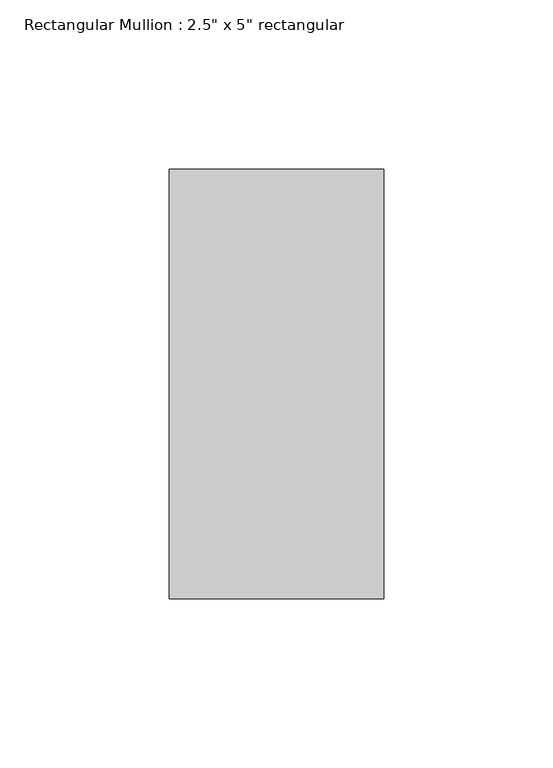
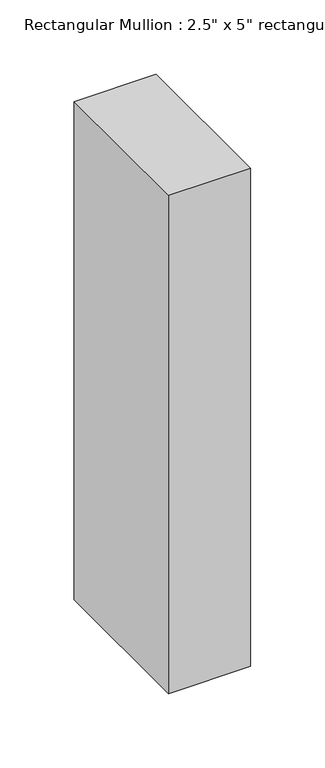
"""IFC4 building model written with IfcOpenShell, lengths in millimetres: member geometry."""

from ifc_helpers import new_model, si_unit, frame, origin, place, context, project, spatial, polyline, outline, extrude, source, transform, mapped, element, save


def member_909e4c35(model_context):
    return source(origin(), model_context, "Body", "SweptSolid", [
        extrude(outline(polyline([(0.0, 63.5), (0.0, -63.5), (-63.5, -63.5), (-63.5, 63.5), (0.0, 63.5)])), frame((0.0, 0.0, -408.5166667), z_axis=(0.0, 0.0, 1.0), x_axis=(1.0, 0.0, 0.0)), (0.0, 0.0, 1.0), 408.5166667),
    ])


if __name__ == "__main__":
    model = new_model("IFC4")
    model_context = context("Model", 3, world=origin())
    ifc_project = project(units=[si_unit("LENGTHUNIT", "METRE", prefix="MILLI")], contexts=[model_context])
    site = spatial("IfcSite", under=ifc_project)
    building = spatial("IfcBuilding", under=site)
    placement = place(None, origin())
    member_shape = member_909e4c35(model_context)
    element("IfcMember", 1, ObjectType="Rectangular Mullion : 2.5\" x 5\" rectangular", at=placement, inside=building, context=model_context, shape_type="MappedRepresentation", body=[
        mapped(member_shape, transform((0.0, 0.0, 0.0), x_axis=(1.0, 0.0, 0.0), y_axis=(0.0, 1.0, 0.0), z_axis=(0.0, 0.0, 1.0))),
    ])
    save(model, "model.ifc")

# Revit data of these elements
# Type "Rectangular Mullion : 2.5\" x 5\" rectangular"
#   built-in parameter 1007304 = 0.416667 (stored number, unit not read)
#   built-in parameter 1007301 = 0.104167 (stored number, unit not read)
#   built-in parameter 1007300 = 0.104167 (stored number, unit not read)
# Element 1 (IfcMember, "Rectangular Mullion : 2.5\" x 5\" rectangular")
#   Materials on its faces: "Aluminum"
# Materials
#   "Aluminum": class "Metal", colour RGB 247 247 247, transparency 0, Description = "Aluminum 6061", Cost = 0
